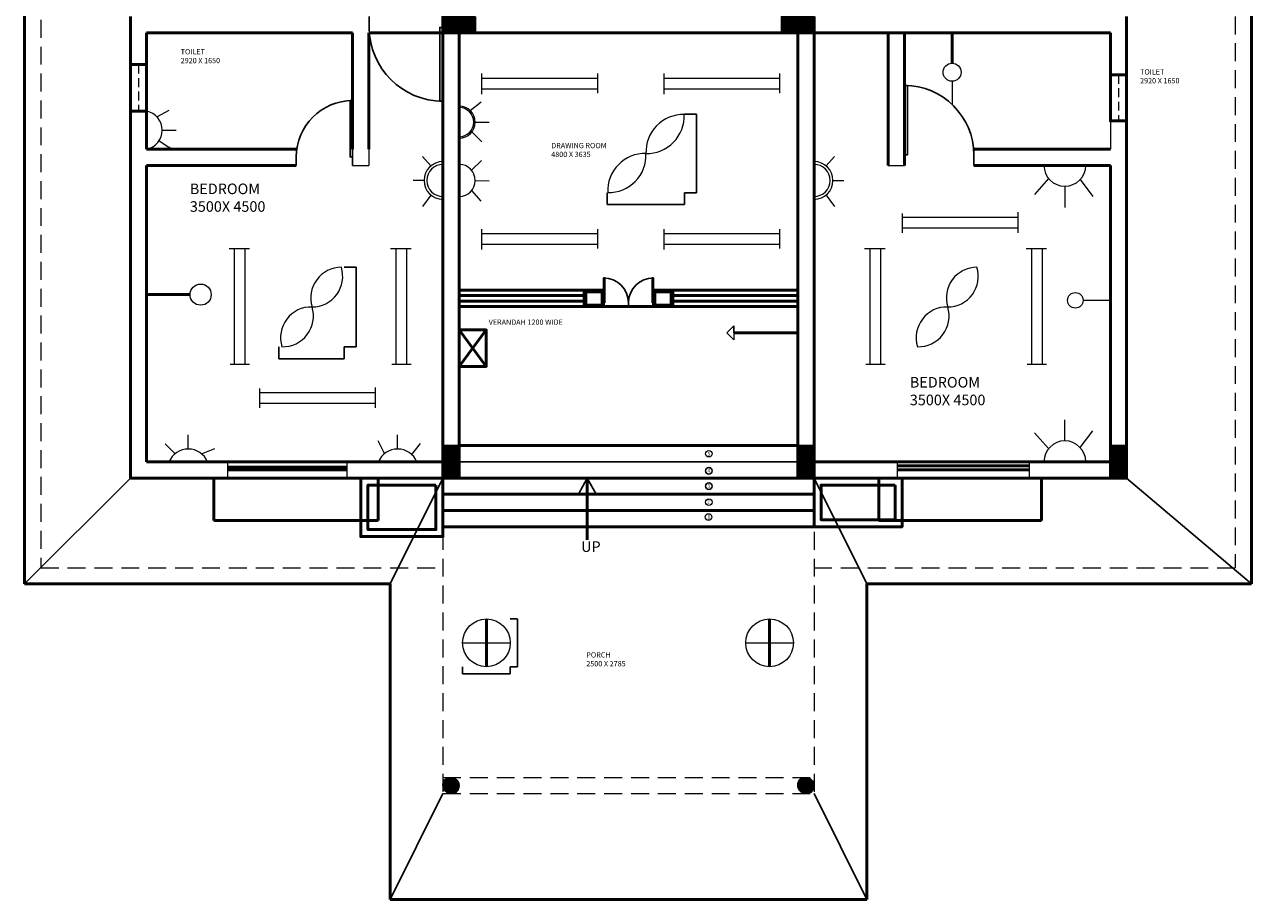
# Model space of a CAD drawing. Units: millimetres. Extents: x 15 to 330868, y -4710 to 1734924.
# Tile 2 of 3: x 311978 to 329368, y 844259 to 856654. Entities that reach past the tile are written whole.
import ezdxf

# ---------------------------------------------------------------- set-up
doc = ezdxf.new("R2010")
doc.units = ezdxf.units.MM
doc.header["$MEASUREMENT"] = 0
doc.linetypes.add('DASHED', pattern=[19.049999999999997, 12.7, -6.349999999999999])
for name, color, linetype, lineweight in [('A-ANNO-DIMS', 2, 'Continuous', 18), ('A-ANNO-TEXT', 7, 'Continuous', 18), ('A-AREA-IDEN', 30, 'Continuous', 25), ('A-COLS', 8, 'Continuous', 35), ('A-DOOR', 4, 'Continuous', 25), ('A-FLOR-STRS', 3, 'Continuous', 25), ('A-ROOF', 6, 'Continuous', 25), ('A-ROOF-OVHD', 6, 'DASHED', 18), ('A-WALL', 7, 'Continuous', 50), ('E-LITE', 1, 'Continuous', 18)]:
    doc.layers.add(name, color=color, linetype=linetype, lineweight=lineweight)
doc.styles.get("Standard").update_dxf_attribs({"font": 'arial.ttf'})
doc.dimstyles.get("Standard").update_dxf_attribs({"dimtxt": 0.18, "dimasz": 0.18, "dimexe": 0.18, "dimexo": 0.0625, "dimgap": 0.09, "dimtad": 0, "dimtih": 1, "dimtoh": 1, "dimdec": 0, "dimzin": 0, "dimdsep": 46, "dimtxsty": 'Standard', "dimcen": 0.09, "dimadec": 0, "dimazin": 0, "dimtfac": 1, "dimtdec": 0, "dimtofl": 0, "dimtmove": 0, "dimatfit": 3, "dimfxl": 1, "dimtolj": 1, "dimtzin": 0, "dimarcsym": 0})
pattern_1 = [(45, (0, 0), (-0.0883883476483185, 0.0883883476483185), [])]

# ---------------------------------------------------------------- blocks, each defined once
blk = doc.blocks.new('*U5')
for p, q in [((0, 0), (-1e-16, -5.999999999999999)), ((40, -6e-16), (40, -6))]:
    blk.add_line(p, q)
blk.add_lwpolyline([(0, 0), (5.6e-15, 40), (1.750000000000007, 40), (1.749999999999998, -7e-16)], close=True)
blk.add_arc((0, 0), 40, 0, 90)
blk = doc.blocks.new('FAN-CEILING')
blk.add_line((543.2829999999958, 553.5), (543.2829999999958, 553.5))
for centre, radius, start, end in [((555.3863884535967, 1083.047616258962), 529.6859162592511, 268.5279151991481, 2.595751645517247), ((1072.491430036316, 575.9857168442104), 529.6859162592514, 88.52791519914813, 182.5957516455172), ((529.6754217544221, 23.98890125169419), 529.6859162592514, 88.52791519914813, 182.5957516455172), ((14.1405782456859, 529.5110987483058), 529.6859162592514, 268.5279151991481, 2.595751645517247)]:
    blk.add_arc(centre, radius, start, end)
blk = doc.blocks.new('FAN-CEILING-2')
for centre, start, end in [((862.0160000000614, 691.0434999999125), 90, 197.1948221549237), ((447.2660000000032, 996.852499999921), 269.9995321854027, 17.19482215492379), ((434.1581541081541, 128.3455810610903), 88.30758652362942, 197.1948221549237), ((32.51600000006147, 434.3524999999208), 268.2535840890827, 17.19482215492379)]:
    blk.add_arc(centre, 434.1544999999459, start, end)
blk = doc.blocks.new('LIGHT-BULKHEAD')
blk.add_line((5.21346810274e-05, 338.0570000000298), (676.113947865262, 338.0570000000298))
blk.add_circle((338.0569999999716, 338.0570000000298), 338.0569478652968)
blk = doc.blocks.new('LIGHT-FTL')
for p, q in [((0, 289), (0, 0)), ((0, 224.5), (1640, 224.5)), ((1640, 289), (1640, 15)), ((0, 74.5), (1640, 74.5))]:
    blk.add_line(p, q)
blk = doc.blocks.new('*D13')
at = {"layer": 'A-ANNO-DIMS', "color": 0, "lineweight": -2, "transparency": 16777216}
for p, q in [((321333.6086021188, 855383.2734574697), (321500.6836170207, 855383.2734574697)), ((321500.5036170207, 855383.0934574696), (321500.5036170207, 854826.9315387656)), ((321500.5036170207, 854270.4033581245), (321500.5036170207, 854826.5652768284)), ((321333.6086021188, 854270.2233581247), (321500.6836170207, 854270.2233581247))]:
    blk.add_line(p, q, dxfattribs=at)
at = {"layer": 'A-ANNO-DIMS', "color": 0, "transparency": 16777216}
for points in [[(321500.4736170206, 855383.0934574696), (321500.5336170207, 855383.0934574696), (321500.5036170207, 855383.2734574697)], [(321500.4736170206, 854270.4033581245), (321500.5336170207, 854270.4033581245), (321500.5036170207, 854270.2233581247)]]:
    blk.add_solid(points, dxfattribs=at)
at = {"layer": 'Defpoints', "color": 0, "transparency": 16777216}
for p in [(321333.5461021188, 855383.2734574697), (321500.5036170207, 855383.2734574697), (321333.5461021188, 854270.2233581247)]:
    blk.add_point(p, dxfattribs=at)
at = {"layer": 'A-ANNO-DIMS', "color": 0, "transparency": 16777216, "insert": (321500.5036170209, 854826.7484077967), "char_height": 0.18, "attachment_point": 5}
blk.add_mtext('\\A1;CEILING FAN 1113 TYP.', dxfattribs=at)
blk = doc.blocks.new('*D14')
at = {"layer": 'A-ANNO-DIMS', "color": 0, "lineweight": -2, "transparency": 16777216}
for p, q in [((320236.2345515984, 854270.1608581243), (320236.2345515984, 854103.0858432224)), ((321333.5461021187, 854270.1608581243), (321333.5461021187, 854103.0858432224)), ((320236.4145515983, 854103.2658432225), (320784.2308589186, 854103.2658432225)), ((321333.3661021187, 854103.2658432225), (320785.5497947985, 854103.2658432225))]:
    blk.add_line(p, q, dxfattribs=at)
at = {"layer": 'A-ANNO-DIMS', "color": 0, "transparency": 16777216}
for points in [[(320236.4145515983, 854103.2958432223), (320236.4145515983, 854103.2358432224), (320236.2345515984, 854103.2658432225)], [(321333.3661021187, 854103.2958432223), (321333.3661021187, 854103.2358432224), (321333.5461021187, 854103.2658432225)]]:
    blk.add_solid(points, dxfattribs=at)
at = {"layer": 'Defpoints', "color": 0, "transparency": 16777216}
for p in [(320236.2345515984, 854270.2233581243), (321333.5461021187, 854270.2233581243), (321333.5461021187, 854103.2658432225)]:
    blk.add_point(p, dxfattribs=at)
at = {"layer": 'A-ANNO-DIMS', "color": 0, "transparency": 16777216, "insert": (320784.8903268585, 854103.2658432225), "char_height": 0.18, "attachment_point": 5}
blk.add_mtext('\\A1;1097 TYP.', dxfattribs=at)
blk = doc.blocks.new('*D15')
at = {"layer": 'A-ANNO-DIMS', "color": 0, "lineweight": -2, "transparency": 16777216}
for p, q in [((316508.8289231396, 853215.5000000003), (316678.3072336224, 853215.5000000003)), ((316678.1272336224, 853215.3200000003), (316678.1272336224, 852651.1470346354)), ((316678.1272336224, 852086.6079301161), (316678.1272336224, 852650.7808954811)), ((316508.8289231396, 852086.4279301161), (316678.3072336224, 852086.4279301161))]:
    blk.add_line(p, q, dxfattribs=at)
at = {"layer": 'A-ANNO-DIMS', "color": 0, "transparency": 16777216}
for points in [[(316678.0972336224, 853215.3200000003), (316678.1572336224, 853215.3200000003), (316678.1272336224, 853215.5000000003)], [(316678.0972336224, 852086.6079301161), (316678.1572336224, 852086.6079301161), (316678.1272336224, 852086.4279301161)]]:
    blk.add_solid(points, dxfattribs=at)
at = {"layer": 'Defpoints', "color": 0, "transparency": 16777216}
for p in [(316508.7664231396, 853215.5000000003), (316678.1272336224, 853215.5000000003), (316508.7664231396, 852086.4279301161)]:
    blk.add_point(p, dxfattribs=at)
at = {"layer": 'A-ANNO-DIMS', "color": 0, "transparency": 16777216, "insert": (316678.1272336226, 852650.963965058), "char_height": 0.18, "attachment_point": 5}
blk.add_mtext('\\A1;CEILING FAN TYPE 2 1129 TYP.', dxfattribs=at)
blk = doc.blocks.new('*D16')
at = {"layer": 'A-ANNO-DIMS', "color": 0, "lineweight": -2, "transparency": 16777216}
for p, q in [((315583.9576186223, 852086.3654301155), (315583.9576186223, 851916.8871196328)), ((316508.7664231395, 852086.3654301155), (316508.7664231395, 851916.8871196328)), ((315584.1376186223, 851917.0671196328), (316045.7640058741, 851917.0671196328)), ((316508.5864231395, 851917.0671196328), (316046.9600358878, 851917.0671196328))]:
    blk.add_line(p, q, dxfattribs=at)
at = {"layer": 'A-ANNO-DIMS', "color": 0, "transparency": 16777216}
for points in [[(315584.1376186223, 851917.0971196329), (315584.1376186223, 851917.0371196329), (315583.9576186223, 851917.0671196328)], [(316508.5864231395, 851917.0971196329), (316508.5864231395, 851917.0371196329), (316508.7664231395, 851917.0671196328)]]:
    blk.add_solid(points, dxfattribs=at)
at = {"layer": 'Defpoints', "color": 0, "transparency": 16777216}
for p in [(315583.9576186223, 852086.4279301155), (316508.7664231395, 852086.4279301155), (316508.7664231395, 851917.0671196328)]:
    blk.add_point(p, dxfattribs=at)
at = {"layer": 'A-ANNO-DIMS', "color": 0, "transparency": 16777216, "insert": (316046.3620208809, 851917.0671196328), "char_height": 0.18, "attachment_point": 5}
blk.add_mtext('\\A1;925 TYP.', dxfattribs=at)
blk = doc.blocks.new('*D19')
at = {"layer": 'A-ANNO-DIMS', "color": 0, "lineweight": -2, "transparency": 16777216}
for p, q in [((318186.4430521348, 847556.3805521348), (318186.4430521348, 847454.8459677752)), ((318186.6230521348, 847455.0259677751), (318522.7880968623, 847455.0259677751)), ((318862.3769478654, 847455.0259677751), (318526.2119031379, 847455.0259677751)), ((318862.5569478654, 847556.3805521348), (318862.5569478654, 847454.8459677752))]:
    blk.add_line(p, q, dxfattribs=at)
at = {"layer": 'A-ANNO-DIMS', "color": 0, "transparency": 16777216}
for points in [[(318186.6230521348, 847455.055967775), (318186.6230521348, 847454.9959677752), (318186.4430521348, 847455.0259677751)], [(318862.3769478654, 847455.055967775), (318862.3769478654, 847454.9959677752), (318862.5569478654, 847455.0259677751)]]:
    blk.add_solid(points, dxfattribs=at)
at = {"layer": 'Defpoints', "color": 0, "transparency": 16777216}
for p in [(318186.4430521348, 847556.4430521348), (318862.5569478654, 847556.4430521348), (318862.5569478654, 847455.0259677751)]:
    blk.add_point(p, dxfattribs=at)
at = {"layer": 'A-ANNO-DIMS', "color": 0, "transparency": 16777216, "insert": (318524.5000000001, 847455.0259677751), "char_height": 0.18, "attachment_point": 5}
blk.add_mtext('\\A1;BULKHEAD LIGHT 676 TYP.', dxfattribs=at)
blk = doc.blocks.new('*D20')
at = {"layer": 'A-ANNO-DIMS', "color": 0, "lineweight": -2, "transparency": 16777216}
for p, q in [((318862.6194478655, 848232.5569478659), (318964.1540322252, 848232.5569478659)), ((318963.9740322252, 848232.3769478657), (318963.9740322252, 847894.6819031383)), ((318963.9740322252, 847556.6230521353), (318963.9740322252, 847894.3180968625)), ((318862.6194478655, 847556.4430521352), (318964.1540322252, 847556.4430521352))]:
    blk.add_line(p, q, dxfattribs=at)
at = {"layer": 'A-ANNO-DIMS', "color": 0, "transparency": 16777216}
for points in [[(318963.9440322251, 848232.3769478657), (318964.0040322252, 848232.3769478657), (318963.9740322252, 848232.5569478659)], [(318963.9440322251, 847556.6230521353), (318964.0040322252, 847556.6230521353), (318963.9740322252, 847556.4430521352)]]:
    blk.add_solid(points, dxfattribs=at)
at = {"layer": 'Defpoints', "color": 0, "transparency": 16777216}
for p in [(318862.5569478655, 848232.5569478659), (318963.9740322252, 848232.5569478659), (318862.5569478655, 847556.4430521352)]:
    blk.add_point(p, dxfattribs=at)
at = {"layer": 'A-ANNO-DIMS', "color": 0, "transparency": 16777216, "insert": (318963.9740322253, 847894.5000000001), "char_height": 0.18, "attachment_point": 5}
blk.add_mtext('\\A1;676 TYP.', dxfattribs=at)

msp = doc.modelspace()

# ---------------------------------------------------------------- hatches: boundary and pattern name
at = {"layer": 'A-COLS'}
h = msp.add_hatch(dxfattribs=at)
h.set_pattern_fill('ANSI31', color=256, scale=10)
h.set_pattern_definition([(45, (318145, 856621), (-0.8838834764831844, 0.8838834764831844), [])])
h.paths.add_polyline_path([(318357.5, 856769.2884389247), (317907.5, 856769.2884389247), (317907.5, 856539.2884389245), (318357.5, 856539.2884389245)])
h.paths.add_polyline_path([(323167.5, 856769.2884389247), (322717.5000000001, 856769.2884389247), (322717.5000000001, 856539.2884389247), (323167.5, 856539.2884389247)])
h = msp.add_hatch(dxfattribs=at)
h.set_pattern_fill('ANSI31', color=256)
h.set_pattern_definition(pattern_1)
h.paths.add_polyline_path([(318137.5000000001, 850679.2884389247), (317907.5000000001, 850679.2884389247), (317907.5000000001, 850229.2884389246), (318137.5000000001, 850229.2884389246)])
h = msp.add_hatch(dxfattribs=at)
h.set_pattern_fill('ANSI31', color=256)
h.set_pattern_definition(pattern_1)
h.paths.add_polyline_path([(323167.5, 850679.2884389247), (322937.5, 850679.2884389247), (322937.5, 850229.2884389246), (323167.5, 850229.2884389246)])
h = msp.add_hatch(dxfattribs=at)
h.set_pattern_fill('ANSI31', color=256)
h.set_pattern_definition(pattern_1)
h.paths.add_polyline_path([(327597.4948108197, 850679.2884389247), (327367.5, 850679.2884389247), (327367.5, 850229.2884389246), (327597.4948108197, 850229.2884389246)])
h = msp.add_hatch(dxfattribs=at)
h.set_pattern_fill('ANSI31', color=256)
h.set_pattern_definition(pattern_1)
h.paths.add_polyline_path([(318137.5000000001, 845874, 1), (317907.5000000001, 845874, 0.393613717575246), (318014.3601132907, 845759.2884389248), (318030.6398867095, 845759.2884389248, 0.393613717575246)])
h = msp.add_hatch(dxfattribs=at)
h.set_pattern_fill('ANSI31', color=256)
h.set_pattern_definition(pattern_1)
h.paths.add_polyline_path([(323167, 845874, 1), (322937, 845874, 0.393613717575246), (323043.8601132906, 845759.2884389248), (323060.1398867094, 845759.2884389248, 0.393613717575246)])

# ---------------------------------------------------------------- linework, layer by layer
at = {"layer": 'A-FLOR-STRS'}
for p, q in [((318137.5, 850459.2884389246), (322937.5, 850459.2884389246)), ((319950.5, 850229.2884389246), (319828.5, 849999.2884389248)), ((319828.5, 849999.2884389248), (319950.5, 850229.2884389246)), ((319950.5, 850229.2884389246), (319950.5, 850229.2884389246)), ((319950.5, 850229.2884389246), (320078, 849999.2884389248))]:
    msp.add_line(p, q, dxfattribs=at)
for centre in [(321676.5, 850332.7908624205), (321676.5, 850115.7908624206)]:
    msp.add_circle(centre, 46.5, dxfattribs=at)
at = {"layer": 'A-ROOF'}
for p, q in [((313477.5, 850229.2884389246), (311977.5000000001, 848729.2884389246)), ((317157.5000000001, 848729.2884389246), (317907.5000000001, 850229.2884389246)), ((323167.5, 850229.2884389246), (323917.5, 848729.2884389246)), ((327597.4948108197, 850229.2884389246), (329367.5462042677, 848729.2884389246)), ((317157.5000000001, 844259.2884389247), (317907.5000000001, 845759.2884389248)), ((323167.5, 845759.2884389248), (323917.5, 844259.2884389247))]:
    msp.add_line(p, q, dxfattribs=at)
at = {"layer": 'A-ROOF-OVHD', "ltscale": 20}
for p, q in [((312207.5000000001, 859769.2884389248), (312207.5000000001, 848959.2884389246)), ((329137.5462042676, 856769.2884389244), (329137.5462042676, 848959.2884389248)), ((317907.5000000001, 850229.2884389246), (317907.5000000001, 845759.2884389248)), ((323167.5, 850229.2884389246), (323167.5, 845759.2884389248)), ((312207.5000000001, 848959.2884389246), (317907.5000000001, 848959.2884389246)), ((323167.5, 848959.2884389244), (329137.5462042676, 848959.2884389246)), ((317907.5000000001, 845989.2884389246), (323167.5, 845989.2884389246)), ((317907.5000000001, 845759.2884389248), (323167.5, 845759.2884389246))]:
    msp.add_line(p, q, dxfattribs=at)
at = {"layer": 'A-ROOF-OVHD', "ltscale": 10}
for p, q in [((313592.5, 856087), (313592.5, 855426.5000000002)), ((327482.5, 855942.5), (327482.5, 855289))]:
    msp.add_line(p, q, dxfattribs=at)
at = {"layer": 'A-WALL'}
for p, q in [((311977.5000000001, 859769.2884389248), (311977.5000000001, 848729.2884389246)), ((329367.5462042676, 859769.2884389244), (329367.5462042677, 851619.2884389246)), ((313477.5, 856769.2884389245), (313477.5, 856087)), ((327597.5000000001, 856769.2884389245), (327597.5000000001, 855942.5)), ((313707.5, 856539.2884389245), (316627.5, 856539.2884389245)), ((313707.5, 856539.2884389245), (313707.5, 856087)), ((316627.5, 854889.2884389239), (316627.5, 856539.2884389245)), ((316857.5, 854889.2884389239), (316857.5, 856539.2884389245)), ((316857.5, 856539.2884389245), (317907.5, 856539.2884389245)), ((317907.5, 856539.2884389245), (317907.5000000001, 850459.2884389246)), ((318137.5, 856539.2884389245), (318137.5, 850459.2884389246)), ((318137.5, 856539.2884389245), (321177.5462042676, 856539.2884389245)), ((321177.5462042677, 856539.2884389245), (322229.2049794545, 856539.2884389245)), ((322229.2049794546, 856539.2884389245), (327367.5000000001, 856539.2884389247)), ((322937.5, 856539.2884389247), (322937.5, 850459.2884389246)), ((323167.5, 856539.2884389247), (323167.5, 850459.2884389245)), ((324217.5000000001, 854659.2884389246), (324217.5000000001, 856539.2884389247)), ((324447.5000000001, 854659.2884389246), (324447.5000000001, 856539.2884389247)), ((325124.5, 856539.2884389245), (325124.5, 856107)), ((327367.5, 856539.2884389247), (327367.5, 855942.5)), ((313477.5, 855426.5000000003), (313477.5, 850229.2884389246)), ((313707.5, 855426.5000000002), (313707.5, 854889.2884389237)), ((327597.5000000001, 855289), (327597.5000000001, 850229.2884389246)), ((313707.5000000001, 854889.2884389239), (315836.8079551775, 854889.2884389239)), ((325432.5, 854889.2884389248), (327367.5, 854889.2884389248)), ((313707.5000000001, 854659.2884389239), (315829.1587751869, 854659.2884389239)), ((313707.5, 854659.2884389239), (313707.5000000001, 850459.2884389245)), ((325432.5, 854659.2884389246), (327367.5, 854659.2884389246)), ((327367.5, 854659.2884389246), (327367.5, 850229.2884389246)), ((313707.5, 852827.8942194626), (314324, 852827.8942194626)), ((318137.5, 852889.2884389248), (320184.7349081405, 852889.2884389248)), ((318137.5, 852814.2884389245), (319911, 852814.2884389245)), ((320890.2650918595, 852889.2884389248), (322937.5, 852889.2884389247)), ((321164, 852814.2884389245), (322937.5, 852814.2884389245)), ((318137.5, 852734.2884389247), (319911, 852734.2884389247)), ((318137.5, 852659.2884389247), (322937.5, 852659.2884389245)), ((321164, 852734.2884389247), (322937.5, 852734.2884389247)), ((318137.5, 851811.4999999999), (318521.5, 852328.4999999999)), ((318137.5, 852328.4999999999), (318521.5, 851811.4999999999)), ((322937.5, 852287), (322033, 852287)), ((329367.5462042677, 851619.2884389246), (329367.5462042677, 848729.2884389246)), ((318137.5, 850689.2884389246), (322937.5, 850689.2884389246)), ((313707.5, 850459.2884389245), (317907.5, 850459.2884389246)), ((314854, 850384.2884389246), (316545, 850384.2884389246)), ((323167.5, 850459.2884389246), (327367.5000000001, 850459.2884389248)), ((324351.5, 850404.2884389246), (326217.9999999999, 850404.2884389246)), ((313477.5, 850229.2884389246), (327597.5000000001, 850229.2884389246)), ((314662, 850229.2884389246), (314662, 849629.2884389246)), ((314854, 850344.2884389246), (316545, 850344.2884389246)), ((316991, 850229.2884389246), (316991, 849629.2884389248)), ((319950.5, 850229.2884389246), (319950.5, 849353.4999999999)), ((324087, 850229.2884389246), (324087, 849629.2884389246)), ((324351.5, 850344.2884389246), (326217.9999999999, 850344.2884389246)), ((326393, 850229.2884389246), (326393, 849629.2884389246)), ((317907.5000000001, 849999.2884389248), (323167.5, 849999.2884389248)), ((317907.5000000001, 849769.2884389248), (323167.5, 849769.2884389246)), ((314662, 849629.2884389246), (316991, 849629.2884389246)), ((317907.5000000001, 849539.2884389247), (323167.5, 849539.2884389245)), ((324086.9999999999, 849629.2884389246), (326393, 849629.2884389246)), ((311977.5000000001, 848729.2884389246), (317157.5000000001, 848729.2884389246)), ((317157.5000000001, 848729.2884389246), (317157.5000000001, 844259.2884389247)), ((323917.5, 848729.2884389246), (329367.5462042677, 848729.2884389246)), ((323917.5, 848729.2884389246), (323917.5, 844259.2884389247)), ((318524.5, 847556.4430521348), (318524.5, 848232.5569478653)), ((322538, 848232.5569478653), (322538, 847556.4430521348)), ((317157.5000000001, 844259.2884389247), (323917.5, 844259.2884389247))]:
    msp.add_line(p, q, dxfattribs=at)
for points in [[(318357.5, 856769.2884389247), (318357.5, 856539.2884389245), (317907.5, 856539.2884389245), (317907.5, 856769.2884389247)], [(323167.5, 856769.2884389247), (323167.5, 856539.2884389247), (322717.5000000001, 856539.2884389247), (322717.5000000001, 856769.2884389247)], [(313477.5, 856087), (313707.5, 856087), (313707.5, 855426.5000000002), (313477.5, 855426.5000000002)], [(327367.5, 855942.5), (327597.5000000001, 855942.5), (327597.5000000001, 855289), (327367.5, 855289)], [(320184.7349081405, 852888.5857486333), (319911, 852888.5857486333), (319911, 852659.2884389247), (320184.7349081405, 852659.2884389247)], [(320164.7349081405, 852868.5857486333), (319931, 852868.5857486333), (319931, 852679.2884389246), (320164.7349081405, 852679.2884389246)], [(321164, 852889.2884389248), (320890.2650918595, 852889.2884389248), (320890.2650918595, 852659.9911292162), (321164, 852659.9911292162)], [(321144, 852869.2884389249), (320910.2650918595, 852869.2884389249), (320910.2650918595, 852679.9911292162), (321144, 852679.9911292162)], [(318137.5, 852328.4999999999), (318521.5, 852328.4999999999), (318521.5, 851811.4999999999), (318137.5, 851811.4999999999)], [(317907.5000000001, 850229.2884389246), (316744, 850229.2884389246), (316744, 849400), (317907.5000000001, 849400)], [(324415.5, 850229.2884389246), (323167.5, 850229.2884389246), (323167.5, 849539.2884389245), (324415.5, 849539.2884389245)], [(317807.5000000001, 850129.2884389247), (316844, 850129.2884389247), (316844, 849500), (317807.5000000001, 849500)], [(324315.5, 850129.2884389247), (323267.5, 850129.2884389247), (323267.5, 849639.2884389246), (324315.5, 849639.2884389246)]]:
    msp.add_lwpolyline(points, close=True, dxfattribs=at)
for points in [[(317199.2049794545, 856539.2884389245), (316969.2049794545, 856539.2884389245)], [(327367.5, 855942.5), (327597.5000000001, 855942.5)], [(327597.5000000001, 855289), (327367.5, 855289)], [(317907.5000000001, 850679.2884389247), (318137.5000000001, 850679.2884389247), (318137.5000000001, 850229.2884389246), (317907.5000000001, 850229.2884389246), (317907.5000000001, 850679.2884389247)], [(322937.5, 850679.2884389247), (323167.5, 850679.2884389247), (323167.5, 850229.2884389246), (322937.5, 850229.2884389246), (322937.5, 850679.2884389247)], [(327367.4948108197, 850679.2884389247), (327597.4948108197, 850679.2884389247), (327597.4948108197, 850229.2884389246), (327367.4948108197, 850229.2884389246), (327367.4948108197, 850679.2884389247)]]:
    msp.add_lwpolyline(points, dxfattribs=at)
at = {"layer": 'E-LITE'}
for p, q in [((313707.5, 856087), (313477.5, 856086.9999999999)), ((325124.5, 855850), (325123.2162867601, 855523.1990766063)), ((313477.5, 855426.5000000002), (313707.5, 855426.5)), ((313852.5183402955, 855347.0396885801), (314029.2106660557, 855440.7403930465)), ((318291.519597068, 855438.9342071353), (318449.707956868, 855561.3124847168)), ((318365, 855271.5), (318565, 855271.5)), ((327367.5, 855289), (327367.5, 854889.2884389248)), ((313928.3659289684, 855157.894219462), (314128.3659289684, 855157.894219462)), ((318319.2041198068, 855134.6063812838), (318460.9591303139, 854993.5194683678)), ((313883.485456061, 855007.6971183761), (314049.5128614575, 854896.185232654)), ((314049.5128614575, 854896.185232654), (314021.5, 854914.9999999999)), ((316627.5000000001, 854889.2884389241), (316627.5, 854659.2884389239)), ((316857.5000000001, 854889.2884389241), (316857.5, 854659.2884389239)), ((317736.1074431717, 854650.8797494007), (317617, 854786)), ((318311.964066153, 854591.5086970746), (318456.5264588917, 854729.7176497718)), ((323338.8925568284, 854650.8797494007), (323458, 854786)), ((325432.5, 854889.2884389248), (325432.5, 854659.2884389246)), ((316627.5000000001, 854659.2884389239), (316857.5, 854659.2884389239)), ((324217.5000000001, 854659.2884389246), (324447.5000000001, 854659.2884389246)), ((317640, 854445.5000000001), (317483.5, 854445.5000000001)), ((318365, 854445.5000000001), (318564.9579356938, 854441.398298755)), ((323435, 854445.5000000001), (323591.5, 854445.5000000001)), ((326492.1818549791, 854472.6804217491), (326294.5325204325, 854246.9931590307)), ((326939.5273787373, 854457.3772780678), (327121.4864880592, 854218.8591811972)), ((317736.9208003764, 854239.4442146997), (317617, 854078.5000000001)), ((318314.2648868648, 854302.2853891125), (318446.7006398661, 854152.4162084016)), ((323338.0791996237, 854239.4442146997), (323458, 854078.5000000001)), ((326722.5, 854362.8613821296), (326722.5, 854062.8613821295)), ((317907.5000000001, 852889.2884389247), (317907.5000000001, 852659.2884389247)), ((317907.5000000001, 852659.2884389247), (317907.5000000001, 852774.2884389246)), ((320536.8079863156, 852734.2884389247), (320538.1920136844, 852734.2884389247)), ((320537.5, 852659.2884389247), (320537.5, 852734.2884389245)), ((327367.5, 852747), (326982, 852747)), ((321933, 852287), (322033, 852387)), ((321933, 852287), (322033, 852187)), ((322033, 852287), (322033, 852387)), ((322033, 852387), (322033, 852387)), ((322033, 852387), (322033, 852287)), ((322033, 852287), (322033, 852187)), ((326722.5, 850755.7154957195), (326722.5, 851055.7154957195)), ((326939.5273787373, 850661.1995997813), (327121.4864880592, 850899.717696652)), ((314298.25, 850640.9480381852), (314298.25, 850840.9480381855)), ((317079.0125893159, 850575.7294669249), (316990.5171866516, 850755.0854361797)), ((317264.75, 850640.9480381854), (317264.75, 850840.9480381855)), ((326492.1818549791, 850645.8964561003), (326294.5325204325, 850871.5837188185)), ((314111.0859642521, 850574.5794585214), (313970.1572260621, 850716.4917227981)), ((314487.2805913682, 850573.0526980121), (314673.3794066983, 850646.3140857464)), ((317466.7536992715, 850561.7050263662), (317591.2437642138, 850718.2368880769)), ((314854, 850459.2884389245), (314854, 850229.2884389246)), ((316545, 850459.2884389245), (316545, 850229.2884389246)), ((324351.5, 850229.2884389246), (324351.5, 850459.2884389246)), ((326218, 850459.2884389246), (326218, 850229.2884389246)), ((327597.4948108197, 850459.2884389246), (327597.5000000001, 850459.2884389246))]:
    msp.add_line(p, q, dxfattribs=at)
for centre, radius in [((325124.5, 855978.5000000001), 128.5), ((314473.3942194625, 852827.8942194626), 149.3942194625269), ((326871.5, 852747), 110.5), ((321676.5, 850574.5), 46.5), ((321676.5, 849886.2908624206), 46.5), ((321672.8922879668, 849677.7908624205), 46.5), ((318022.5000000001, 845874), 115), ((323052, 845874), 115)]:
    msp.add_circle(centre, radius, dxfattribs=at)
for centre, radius, start, end in [((313654.600698445, 855157.8942194622), 273.765230523407, 281.1412681363048, 78.85873186364448), ((318137.5, 855271.5), 227.5, 270, 90), ((318137.5, 855271.5), 207.5, 270, 90), ((317907.5, 854445.5000000001), 267.5, 90, 270), ((317907.5, 854445.5000000001), 227.5, 90, 270), ((318137.5, 854445.5000000001), 227.5, 270, 90), ((323167.5, 854445.5000000001), 267.5, 270, 90), ((323167.5, 854445.5000000001), 227.5, 270, 90), ((326722.5, 854659.2884389246), 296.4270567948438, 180, 0), ((326722.5, 850459.2884389246), 296.4270567948438, 2.25017e-11, 179.9999999999775), ((314298.25, 850343.855913842), 297.0921243435222, 22.86375788127598, 157.1362421187265), ((317264.75, 850343.8559138421), 297.0921243435222, 22.8637578812766, 157.1362421187263)]:
    msp.add_arc(centre, radius, start, end, dxfattribs=at)

# ---------------------------------------------------------------- block references
at = {"layer": 'A-DOOR', "xscale": 26.10303855837779, "yscale": 26.10303855837779, "zscale": 26.10303855837779, "rotation": 180}
msp.add_blockref('*U5', (317907.5, 856612.6702075743), dxfattribs=at)
at = {"layer": 'A-DOOR'}
for p, xscale, yscale, zscale in [((324447.9279355922, 854806.9474753996), 24.60983941249804, 24.60983941249804, 24.60983941249804), ((316627.4999999999, 854779.039622646), -19.95853062032723, 19.95853062032723, 19.95853062032723), ((320184.7349081405, 852712.2032027035), 8.819127296487046, 8.819127296487046, 8.819127296487046), ((320890.2650918595, 852712.2032027035), -8.819127296487046, 8.819127296487046, 8.819127296487046)]:
    msp.add_blockref('*U5', p, dxfattribs=dict(at, xscale=xscale, yscale=yscale, zscale=zscale))
at = {"layer": 'E-LITE'}
for name, p in [('LIGHT-FTL', (318456.5, 855669.5000000003)), ('LIGHT-FTL', (321037, 855669.5000000003)), ('FAN-CEILING', (320242.3594217545, 854274.0000000003)), ('LIGHT-FTL', (318456.5, 853468.5000000001)), ('LIGHT-FTL', (321037, 853468.5000000001)), ('FAN-CEILING-2', (315605.984, 852090.302)), ('FAN-CEILING-2', (324614.7340000014, 852090.302)), ('LIGHT-BULKHEAD', (318186.4430000001, 847556.443)), ('LIGHT-BULKHEAD', (322199.943, 847556.443))]:
    msp.add_blockref(name, p, dxfattribs=at)
for p, rotation in [((326060.5, 853994.5000000001), 180), ((314876.4202178699, 853478.4892006626), 269.9999999999935), ((317166.5517956894, 853478.4892006626), 270.0000000000014), ((323885.1702178715, 853478.4892006626), 269.9999999999975), ((326175.301795691, 853478.4892006626), 269.9999999999975), ((316954, 851512), 180)]:
    msp.add_blockref('LIGHT-FTL', p, dxfattribs=dict(at, rotation=rotation))

# ---------------------------------------------------------------- texts
at = {"layer": 'A-ANNO-TEXT', "attachment_point": 1}
for s, insert, char_height in [('5', (321657.6473397, 850598.8526603003), 50), ('4', (321658.5, 850361), 50), ('3', (321657.4085948158, 850142.5914051844), 50), ('2', (321652.0000000001, 849921), 50), ('1', (321658.295361528, 849705.7046384718), 50), ('UP', (319866, 849332.704638472), 150)]:
    msp.add_mtext_dynamic_manual_height_columns(s, width=4478, gutter_width=1, heights=[0], dxfattribs=dict(at, insert=insert, char_height=char_height))
at = {"layer": 'A-AREA-IDEN', "char_height": 150, "attachment_point": 1}
for s, insert in [('{\\H0.5x;TOILET\\P2920 X 1650}', (314190.5, 856306.4999999999)), ('{\\H0.5x;TOILET\\P2920 X 1650}', (327788.5, 856021)), ('{\\H0.5x;DRAWING ROOM \\P4800 X 3635}', (319442.5, 854977.3908594815)), ('BEDROOM\\P3500X 4500', (314320, 854401.4999999999)), ('{\\H0.5x;VERANDAH 1200 WIDE}', (318556, 852475.5)), ('BEDROOM\\P3500X 4500', (324525, 851661)), ('{\\H0.5x;PORCH\\P2500 X 2785}', (319939.5, 847761.5))]:
    msp.add_mtext_dynamic_manual_height_columns(s, width=7683.453795732522, gutter_width=1, heights=[0], dxfattribs=dict(at, insert=insert))

# ---------------------------------------------------------------- dimensions: what is measured, and where the dimension line sits
at = {"layer": 'A-ANNO-DIMS'}
for base, p1, p2, text, picture, middle in [((321500.5036170207, 855383.2734574697), (321333.5461021187, 854270.2233581243), (321333.5461021187, 855383.273457469), 'CEILING FAN <> TYP.', '*D13', (321500.5036170209, 854826.7484077967)), ((316678.1272336224, 853215.5000000003), (316508.7664231395, 852086.4279301155), (316508.7664231395, 853215.4999999999), 'CEILING FAN TYPE 2 <> TYP.', '*D15', (316678.1272336226, 852650.963965058)), ((318963.9740322252, 848232.5569478659), (318862.5569478654, 847556.4430521348), (318862.5569478654, 848232.5569478653), '<> TYP.', '*D20', (318963.9740322253, 847894.5000000001))]:
    dim = msp.add_linear_dim(base=base, p1=p1, p2=p2, angle=90, text=text, dimstyle='Standard', override={"dimdec": 0, "dimlfac": 1, "dimrnd": 0, "dimzin": 0, "dimdsep": 46, "dimlunit": 2}, dxfattribs=at)
    dim.commit()
    dim.dimension.update_dxf_attribs({"geometry": picture, "text_midpoint": middle})
for base, p1, p2, text, picture, middle in [((321333.5461021187, 854103.2658432225), (320236.2345515984, 854270.2233581243), (321333.5461021187, 854270.2233581243), '<> TYP.', '*D14', (320784.8903268585, 854103.2658432225)), ((316508.7664231395, 851917.0671196328), (315583.9576186223, 852086.4279301155), (316508.7664231395, 852086.4279301155), '<> TYP.', '*D16', (316046.3620208809, 851917.0671196328)), ((318862.5569478654, 847455.0259677751), (318186.4430521348, 847556.4430521348), (318862.5569478654, 847556.4430521348), 'BULKHEAD LIGHT <> TYP.', '*D19', (318524.5000000001, 847455.0259677751))]:
    dim = msp.add_linear_dim(base=base, p1=p1, p2=p2, text=text, dimstyle='Standard', override={"dimdec": 0, "dimlfac": 1, "dimrnd": 0, "dimzin": 0, "dimdsep": 46, "dimlunit": 2}, dxfattribs=at)
    dim.commit()
    dim.dimension.update_dxf_attribs({"geometry": picture, "text_midpoint": middle})

doc.saveas('drawing.dxf')
